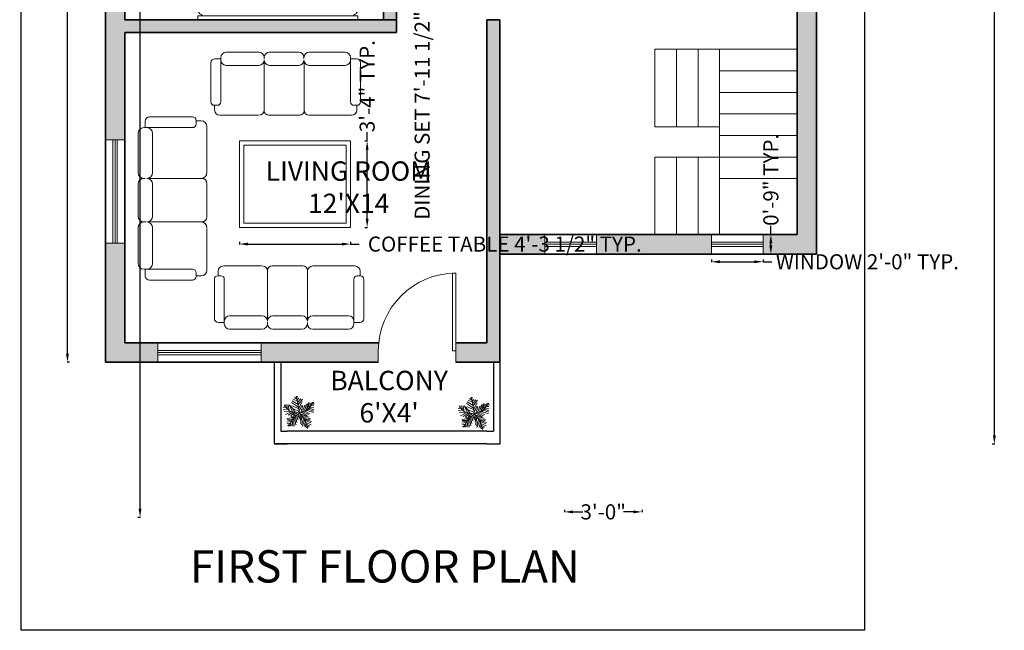
# Model space of a CAD drawing. Units: inches. Extents: x -80 to 1461, y -1239 to 153.
# Tile 4 of 6: x 358 to 815, y -556 to -273. Entities that reach past the tile are written whole.
import ezdxf

# ---------------------------------------------------------------- set-up
doc = ezdxf.new("R2010")
doc.units = ezdxf.units.IN
doc.header["$MEASUREMENT"] = 0
for name, color, linetype, lineweight in [('A-ANNO-DIMS', 2, 'Continuous', 18), ('A-ANNO-TEXT', 7, 'Continuous', 18), ('A-ANNO-TTLB', 7, 'Continuous', 25), ('A-AREA-IDEN', 7, 'Continuous', 18), ('A-FLOR', 7, 'Continuous', 25), ('A-FLOR-STRS', 7, 'Continuous', 20), ('A-FURN', 8, 'Continuous', 18), ('A-GLAZ', 4, 'Continuous', 18), ('A-WALL', 7, 'Continuous', 35), ('A-WALL-PATT', 8, 'Continuous', 13), ('DOOR', 32, 'Continuous', 18), ('TREE', 92, 'Continuous', 13)]:
    doc.layers.add(name, color=color, linetype=linetype, lineweight=lineweight)
doc.styles.get("Standard").update_dxf_attribs({"font": 'arial.ttf'})
doc.dimstyles.get("Standard").update_dxf_attribs({"dimtxt": 7, "dimasz": 4, "dimexe": 0.18, "dimexo": 0.0625, "dimgap": 0.09, "dimtad": 0, "dimdec": 0, "dimzin": 0, "dimdsep": 46, "dimlunit": 3, "dimtxsty": 'Standard', "dimcen": 0.09, "dimadec": 0, "dimazin": 0, "dimtfac": 1, "dimtdec": 0, "dimtofl": 0, "dimtmove": 0, "dimatfit": 3, "dimfxl": 1, "dimfxlon": 1, "dimtolj": 1, "dimtzin": 0, "dimarcsym": 0})

# ---------------------------------------------------------------- blocks, each defined once
blk = doc.blocks.new('*U10')
for p, q in [((-3.665, 19.273), (-27.574, 35.527)), ((-5.114, 28.097), (-24.676, 40.636)), ((-7.288, 39.707), (-21.778, 46.673)), ((-8.737, 47.138), (-17.069, 52.711)), ((-10.186, 53.64), (-13.084, 55.962)), ((0, 0), (-10.5, 57)), ((-9.099, 51.782), (-6.563, 55.962)), ((-7.65, 43.423), (-2.578, 49.46)), ((-5.839, 35.992), (4.667, 48.067)), ((-5.114, 27.632), (10.463, 46.673)), ((-2.941, 16.486), (8.652, 37.85)), ((27, 9), (48, 36)), ((27.127, 9.056), (31.112, 35.992)), ((38.719, 34.134), (41.979, 28.561)), ((44.153, 36.456), (45.239, 32.741)), ((-47.498, 19.737), (-55.83, 18.344)), ((-40.615, 13.7), (-55.105, 10.913)), ((-31.5, 4.5), (-52.5, 25.5)), ((-33.37, 6.269), (-52.207, 5.34)), ((-48.585, 21.131), (-49.309, 29.026)), ((-28.299, 3.483), (-47.86, -5.805)), ((-43.513, 28.561), (-42.427, 15.558)), ((-38.442, 26.239), (-34.819, 7.663)), ((-21.416, 3.018), (-38.079, -8.128)), ((-35.544, 28.097), (-24.314, 3.947)), ((0, 0), (-31.5, 4.5)), ((-14.533, 2.09), (-30.834, 25.31)), ((-15.982, 2.09), (-30.11, -9.521)), ((-24.314, 23.917), (-2.941, 13.7)), ((0, 0), (-22.5, -19.5)), ((-6.563, 1.161), (-21.416, -8.128)), ((-20.691, 13.7), (-1.129, 4.876)), ((-1.129, 6.734), (9.014, 26.704)), ((0, 0), (27, 9)), ((0, 0), (18, -22.5)), ((3.942, 1.625), (11.187, 24.381)), ((6.478, 1.625), (26.04, -8.592)), ((10.101, 3.483), (17.708, 26.239)), ((11.187, 3.483), (30.749, -5.805)), ((16.259, 5.805), (23.142, 31.348)), ((18.07, 5.805), (35.096, -3.483)), ((22.055, 7.198), (27.489, 32.277)), ((24.229, 7.663), (46.688, 1.625)), ((29.662, 12.307), (48.137, 6.269)), ((31.836, 30.883), (32.561, 16.486)), ((33.285, 16.486), (48.862, 10.913)), ((35.096, 32.741), (37.27, 22.524)), ((36.183, 19.737), (48.137, 17.88)), ((40.53, 25.775), (48.862, 24.846)), ((43.791, 29.954), (51.036, 30.883)), ((-17.431, -15.094), (-42.789, -18.809)), ((-28.299, -29.026), (-42.789, -31.348)), ((-24.314, -21.596), (-42.427, -22.06)), ((-26.849, -26.24), (-40.253, -25.775)), ((-22.5, -19.5), (-37.5, -45)), ((-15.257, -12.772), (-30.11, -12.772)), ((-29.023, -30.884), (-27.936, -43.887)), ((-25.038, -23.918), (-22.865, -45.281)), ((-20.691, -18.345), (-17.793, -44.352)), ((-6.563, -5.805), (-19.967, -9.985)), ((-17.069, -15.094), (-12.721, -40.172)), ((-13.446, -11.378), (-8.737, -32.741)), ((-9.461, -8.592), (-6.201, -23.453)), ((-4.752, -3.483), (-3.665, -14.629)), ((2.493, -3.019), (-1.491, -20.202)), ((1.769, -2.555), (24.229, -9.521)), ((5.029, -6.27), (2.131, -25.775)), ((9.014, -11.378), (3.58, -35.992)), ((14.085, -16.951), (6.478, -40.172)), ((7.565, -9.056), (32.198, -14.629)), ((18.07, -22.524), (8.289, -45.745)), ((12.274, -15.094), (36.907, -18.809)), ((20.244, -30.419), (15.897, -44.816)), ((16.259, -19.738), (36.183, -22.989)), ((18, -22.5), (27, -52.5)), ((18.433, -22.524), (40.53, -29.026)), ((19.157, -25.311), (38.719, -33.206)), ((21.331, -32.741), (39.081, -40.636)), ((-30.834, -34.135), (-42.427, -35.528)), ((-34.457, -39.708), (-40.978, -42.494)), ((-32.646, -36.921), (-31.921, -44.352)), ((22.78, -37.85), (19.519, -48.532)), ((22.78, -38.314), (34.372, -44.816)), ((24.591, -45.745), (23.142, -50.854)), ((24.591, -43.423), (30.749, -47.603)), ((26.764, -49.925), (28.213, -50.854))]:
    blk.add_line(p, q)
blk = doc.blocks.new('*U2')
for p, q in [((0, 0), (0, -6)), ((40, 0), (40, -6))]:
    blk.add_line(p, q)
blk.add_lwpolyline([(0, 0), (0, 40), (1.75, 40), (1.75, 0)], close=True)
blk.add_arc((0, 0), 40, 0, 90)
blk = doc.blocks.new('A$C164346CA')
for p, q in [((0, 2.035), (0, 2)), ((1.5, 2.035), (0, 2.035)), ((1.5, 2), (1.5, 2.035)), ((1.5, 2), (0, 2)), ((0, 1.93), (0, 0.07)), ((0.0919, 1.8624), (0.0919, 1.6069)), ((0.6731, 1.9024), (0.1319, 1.9024)), ((0.7131, 1.6069), (0.7131, 1.8624)), ((0.7828, 1.8624), (0.7828, 1.6069)), ((1.364, 1.9024), (0.8228, 1.9024)), ((1.404, 1.6069), (1.404, 1.8624)), ((1.5, 0.07), (1.5, 1.93)), ((0.1319, 1.5669), (0.6731, 1.5669)), ((0.8228, 1.5669), (1.364, 1.5669)), ((0.8395, 1.4761), (0, 1.4761)), ((0.8395, 1.4761), (1.2448, 1.12)), ((1.5, 1.2611), (0.8395, 1.4761)), ((1.3077, 1.1175), (1.5, 1.2611)), ((0.07, 0), (1.43, 0))]:
    blk.add_line(p, q)
for centre, radius, start, end in [((0.07, 1.93), 0.07, 90, 180), ((1.43, 1.93), 0.07, 0, 90), ((0.1319, 1.8624), 0.04, 90, 180), ((0.6731, 1.8624), 0.04, 0, 90), ((0.8228, 1.8624), 0.04, 90, 180), ((1.364, 1.8624), 0.04, 0, 90), ((0.1319, 1.6069), 0.04, 180, 270), ((0.6731, 1.6069), 0.04, 270, 0), ((0.8228, 1.6069), 0.04, 180, 270), ((1.364, 1.6069), 0.04, 270, 0), ((1.2778, 1.1575), 0.05, 228.69584, 306.75789), ((0.07, 0.07), 0.07, 180, 270), ((1.43, 0.07), 0.07, 270, 0)]:
    blk.add_arc(centre, radius, start, end)
blk = doc.blocks.new('A$C0876780F')
for p, q in [((0.72, 0.95), (0.23, 0.95)), ((1.32, 0.95), (0.88, 0.95)), ((1.48, 0.95), (2.02, 0.95)), ((0.15, 0.85), (0.06, 0.85)), ((0.15, 0.87), (0.15, 0.844)), ((0.15, 0.87), (0.15, 0.85)), ((0.15, 0.21), (0.15, 0.85)), ((0.8, 0.85), (0.8, 0.87)), ((0.8, 0.87), (0.8, 0.85)), ((0.8, 0.87), (0.8, 0.844)), ((0.801, 0.82), (0.801, 0.08)), ((1.4, 0.85), (1.4, 0.87)), ((1.4, 0.85), (1.4, 0.87)), ((2.1, 0.87), (2.1, 0.85)), ((2.1, 0.87), (2.1, 0.844)), ((2.1, 0.21), (2.1, 0.85)), ((2.1, 0.85), (2.19, 0.85)), ((0, 0.79), (0, 0.21)), ((0.72, 0.75), (0.23, 0.75)), ((1.32, 0.75), (0.88, 0.75)), ((1.401, 0.08), (1.401, 0.803)), ((1.48, 0.75), (2.02, 0.75)), ((2.25, 0.79), (2.25, 0.21)), ((0, 0.21), (0, 0.2)), ((0.05, 0.15), (0.1, 0.15)), ((0.056, 0.15), (0.056, 0.08)), ((0.15, 0.2), (0.15, 0.25)), ((2.1, 0.2), (2.1, 0.25)), ((2.2, 0.15), (2.15, 0.15)), ((2.194, 0.15), (2.194, 0.08)), ((2.25, 0.21), (2.25, 0.2)), ((0.136, 0), (0.709, 0)), ((0.801, 0.07), (0.801, 0.08)), ((0.871, 0), (1.331, 0)), ((1.401, 0.07), (1.401, 0.08)), ((2.114, 0), (1.48, 0))]:
    blk.add_line(p, q)
for centre, radius, start, end in [((0.23, 0.87), 0.08, 90, 180), ((0.72, 0.87), 0.08, 0, 90), ((0.88, 0.87), 0.08, 90, 180), ((1.32, 0.87), 0.08, 0, 90), ((1.48, 0.87), 0.08, 90, 180), ((2.02, 0.87), 0.08, 0, 90), ((0.06, 0.79), 0.06, 90, 180), ((0.23, 0.83), 0.08, 180, 270), ((0.23, 0.83), 0.08, 180, 270), ((0.72, 0.83), 0.08, 270, 0), ((0.88, 0.83), 0.08, 180, 270), ((0.88, 0.83), 0.08, 180, 270), ((1.32, 0.83), 0.08, 270, 0), ((1.48, 0.83), 0.08, 180, 270), ((2.02, 0.83), 0.08, 270, 0), ((2.02, 0.83), 0.08, 270, 0), ((2.19, 0.79), 0.06, 0, 90), ((0.05, 0.2), 0.05, 180, 270), ((0.1, 0.2), 0.05, 270, 0), ((0.09, 0.21), 0.06, 350.5377, 0), ((2.16, 0.21), 0.06, 180, 189.4623), ((2.15, 0.2), 0.05, 180, 270), ((2.2, 0.2), 0.05, 270, 0), ((0.136, 0.08), 0.08, 180, 270), ((0.721, 0.08), 0.08, 270, 0), ((0.871, 0.07), 0.07, 180, 270), ((1.331, 0.07), 0.07, 270, 0), ((1.481, 0.08), 0.08, 180, 270), ((2.114, 0.08), 0.08, 270, 0)]:
    blk.add_arc(centre, radius, start, end)
blk = doc.blocks.new('*D14')
at = {"layer": 'A-ANNO-DIMS', "color": 0, "lineweight": -2, "transparency": 16777216}
for p, q in [((380.82, 30.32), (379.64, 30.32)), ((379.82, 26.32), (379.82, -188.57)), ((379.82, -427.68), (379.82, -212.8)), ((380.82, -431.68), (379.64, -431.68))]:
    blk.add_line(p, q, dxfattribs=at)
at = {"layer": 'A-ANNO-DIMS', "color": 0, "transparency": 16777216}
for points in [[(379.15, 26.32), (380.48, 26.32), (379.82, 30.32)], [(379.15, -427.68), (380.48, -427.68), (379.82, -431.68)]]:
    blk.add_solid(points, dxfattribs=at)
at = {"layer": 'Defpoints', "color": 0, "transparency": 16777216}
for p in [(397.42, 30.32), (379.82, -431.68), (397.42, -431.68)]:
    blk.add_point(p, dxfattribs=at)
at = {"layer": 'A-ANNO-DIMS', "color": 0, "transparency": 16777216, "insert": (379.82, -200.68), "char_height": 7, "attachment_point": 5, "rotation": 90}
blk.add_mtext('\\A1;38\'-6"', dxfattribs=at)
blk = doc.blocks.new('WIN-48IN')
for p, q in [((0, 9), (0, 0)), ((48, 9), (0, 9)), ((0, 5.5), (48, 5.5)), ((48, 0), (48, 9)), ((0, 4.5), (48, 4.5)), ((0, 3.5), (48, 3.5)), ((0, 0), (36, 0)), ((36, 0), (48, 0))]:
    blk.add_line(p, q)
blk = doc.blocks.new('WIN-24IN')
for p, q in [((0, 9), (0, 0)), ((0, 9), (24, 9)), ((0, 5.5), (24, 5.5)), ((24, 9), (24, 0)), ((0, 4.5), (24, 4.5)), ((0, 3.5), (24, 3.5)), ((0, 0), (24, 0))]:
    blk.add_line(p, q)
blk = doc.blocks.new('COFFEE-TABLE')
for points in [[(0, 40.15), (51.49, 40.15), (51.49, 0), (0, 0)], [(2, 38.15), (49.49, 38.15), (49.49, 2), (2, 2)]]:
    blk.add_lwpolyline(points, close=True)
blk = doc.blocks.new('STAIR-RETURN-PLAN')
for p, q in [((0, 86), (0, 50)), ((0, 86), (30, 86)), ((10, 86), (10, 50)), ((20, 86), (20, 50)), ((66, 86), (30, 86)), ((30, 86), (30, 50)), ((66, 76), (30, 76)), ((66, 66), (30, 66)), ((66, 56), (30, 56)), ((0, 50), (30, 50)), ((30, 50), (30, 36)), ((66, 46), (30, 46)), ((0, 36), (0, 0)), ((0, 36), (30, 36)), ((10, 36), (10, 0)), ((20, 36), (20, 0)), ((66, 36), (30, 36)), ((30, 36), (30, 0)), ((66, 26), (30, 26))]:
    blk.add_line(p, q)
blk = doc.blocks.new('*D38')
at = {"layer": 'A-ANNO-DIMS', "color": 0, "lineweight": -2, "transparency": 16777216}
for p, q in [((678.59, -384.02), (678.59, -385.2)), ((682.59, -385.02), (698.59, -385.02)), ((702.59, -384.02), (702.59, -385.2)), ((702.59, -385.02), (706.59, -385.02))]:
    blk.add_line(p, q, dxfattribs=at)
at = {"layer": 'A-ANNO-DIMS', "color": 0, "transparency": 16777216}
for points in [[(682.59, -384.36), (682.59, -385.69), (678.59, -385.02)], [(698.59, -384.36), (698.59, -385.69), (702.59, -385.02)]]:
    blk.add_solid(points, dxfattribs=at)
at = {"layer": 'Defpoints', "color": 0, "transparency": 16777216}
for p in [(678.59, -381.42), (702.59, -381.42), (702.59, -385.02)]:
    blk.add_point(p, dxfattribs=at)
at = {"layer": 'A-ANNO-DIMS', "color": 0, "transparency": 16777216, "insert": (750.97, -385.02), "char_height": 7, "attachment_point": 5}
blk.add_mtext('\\A1;WINDOW 2\'-0" TYP.', dxfattribs=at)
blk = doc.blocks.new('*D39')
at = {"layer": 'A-ANNO-DIMS', "color": 0, "lineweight": -2, "transparency": 16777216}
for p, q in [((706.19, -372.42), (706.19, -368.42)), ((705.19, -372.42), (706.37, -372.42)), ((706.19, -377.42), (706.19, -376.42)), ((705.19, -381.42), (706.37, -381.42))]:
    blk.add_line(p, q, dxfattribs=at)
at = {"layer": 'A-ANNO-DIMS', "color": 0, "transparency": 16777216}
for points in [[(705.52, -376.42), (706.86, -376.42), (706.19, -372.42)], [(705.52, -377.42), (706.86, -377.42), (706.19, -381.42)]]:
    blk.add_solid(points, dxfattribs=at)
at = {"layer": 'Defpoints', "color": 0, "transparency": 16777216}
for p in [(702.59, -372.42), (706.19, -372.42), (702.59, -381.42)]:
    blk.add_point(p, dxfattribs=at)
at = {"layer": 'A-ANNO-DIMS', "color": 0, "transparency": 16777216, "insert": (706.19, -347), "char_height": 7, "attachment_point": 5, "rotation": 90}
blk.add_mtext('\\A1;0\'-9" TYP.', dxfattribs=at)
blk = doc.blocks.new('*D52')
at = {"layer": 'A-ANNO-DIMS', "color": 0, "lineweight": -2, "transparency": 16777216}
for p, q in [((545.39, -145.12), (544.21, -145.12)), ((544.39, -149.12), (544.39, -236.86)), ((545.39, -240.86), (544.21, -240.86)), ((544.39, -240.86), (544.39, -244.86))]:
    blk.add_line(p, q, dxfattribs=at)
at = {"layer": 'A-ANNO-DIMS', "color": 0, "transparency": 16777216}
for points in [[(543.72, -149.12), (545.06, -149.12), (544.39, -145.12)], [(543.72, -236.86), (545.06, -236.86), (544.39, -240.86)]]:
    blk.add_solid(points, dxfattribs=at)
at = {"layer": 'Defpoints', "color": 0, "transparency": 16777216}
for p in [(558.75, -145.12), (544.39, -240.86), (558.75, -240.86)]:
    blk.add_point(p, dxfattribs=at)
at = {"layer": 'A-ANNO-DIMS', "color": 0, "transparency": 16777216, "insert": (544.39, -306.33), "char_height": 7, "attachment_point": 5, "rotation": 90}
blk.add_mtext('\\A1;DINING SET 7\'-11 1/2" TYP.', dxfattribs=at)
blk = doc.blocks.new('*D54')
at = {"layer": 'A-ANNO-DIMS', "color": 0, "lineweight": -2, "transparency": 16777216}
for p, q in [((459.66, -375.81), (459.66, -376.99)), ((463.66, -376.81), (507.15, -376.81)), ((511.15, -375.81), (511.15, -376.99)), ((511.15, -376.81), (515.15, -376.81))]:
    blk.add_line(p, q, dxfattribs=at)
at = {"layer": 'A-ANNO-DIMS', "color": 0, "transparency": 16777216}
for points in [[(463.66, -376.15), (463.66, -377.48), (459.66, -376.81)], [(507.15, -376.15), (507.15, -377.48), (511.15, -376.81)]]:
    blk.add_solid(points, dxfattribs=at)
at = {"layer": 'Defpoints', "color": 0, "transparency": 16777216}
for p in [(459.66, -369.09), (511.15, -369.09), (511.15, -376.81)]:
    blk.add_point(p, dxfattribs=at)
at = {"layer": 'A-ANNO-DIMS', "color": 0, "transparency": 16777216, "insert": (582.73, -376.81), "char_height": 7, "attachment_point": 5}
blk.add_mtext('\\A1;COFFEE TABLE 4\'-3 1/2" TYP.', dxfattribs=at)
blk = doc.blocks.new('*D55')
at = {"layer": 'A-ANNO-DIMS', "color": 0, "lineweight": -2, "transparency": 16777216}
for p, q in [((517.87, -328.94), (519.05, -328.94)), ((518.87, -328.94), (518.87, -324.94)), ((518.87, -365.09), (518.87, -332.94)), ((517.87, -369.09), (519.05, -369.09))]:
    blk.add_line(p, q, dxfattribs=at)
at = {"layer": 'A-ANNO-DIMS', "color": 0, "transparency": 16777216}
for points in [[(518.21, -332.94), (519.54, -332.94), (518.87, -328.94)], [(518.21, -365.09), (519.54, -365.09), (518.87, -369.09)]]:
    blk.add_solid(points, dxfattribs=at)
at = {"layer": 'Defpoints', "color": 0, "transparency": 16777216}
for p in [(511.15, -328.94), (518.87, -328.94), (511.15, -369.09)]:
    blk.add_point(p, dxfattribs=at)
at = {"layer": 'A-ANNO-DIMS', "color": 0, "transparency": 16777216, "insert": (518.87, -303.51), "char_height": 7, "attachment_point": 5, "rotation": 90}
blk.add_mtext('\\A1;3\'-4" TYP.', dxfattribs=at)
blk = doc.blocks.new('*D72')
at = {"layer": 'A-ANNO-DIMS', "color": 0, "lineweight": -2, "transparency": 16777216}
for p, q in [((412.49, 30.32), (413.67, 30.32)), ((413.49, 26.32), (413.49, -224.38)), ((413.49, -499.58), (413.49, -248.89)), ((412.49, -503.58), (413.67, -503.58))]:
    blk.add_line(p, q, dxfattribs=at)
at = {"layer": 'A-ANNO-DIMS', "color": 0, "transparency": 16777216}
for points in [[(412.82, 26.32), (414.16, 26.32), (413.49, 30.32)], [(412.82, -499.58), (414.16, -499.58), (413.49, -503.58)]]:
    blk.add_solid(points, dxfattribs=at)
at = {"layer": 'Defpoints', "color": 0, "transparency": 16777216}
for p in [(330.99, 30.32), (183.99, -503.58), (413.49, -503.58)]:
    blk.add_point(p, dxfattribs=at)
at = {"layer": 'A-ANNO-DIMS', "color": 0, "transparency": 16777216, "insert": (413.49, -236.63), "char_height": 7, "attachment_point": 5, "rotation": 90}
blk.add_mtext('\\A1;44\'-6"', dxfattribs=at)
blk = doc.blocks.new('*D73')
at = {"layer": 'A-ANNO-DIMS', "color": 0, "lineweight": -2, "transparency": 16777216}
for p, q in [((808.92, 30.32), (810.1, 30.32)), ((809.92, 26.32), (809.92, -207.38)), ((809.92, -465.58), (809.92, -231.89)), ((808.92, -469.58), (810.1, -469.58))]:
    blk.add_line(p, q, dxfattribs=at)
at = {"layer": 'A-ANNO-DIMS', "color": 0, "transparency": 16777216}
for points in [[(809.25, 26.32), (810.58, 26.32), (809.92, 30.32)], [(809.25, -465.58), (810.58, -465.58), (809.92, -469.58)]]:
    blk.add_solid(points, dxfattribs=at)
at = {"layer": 'Defpoints', "color": 0, "transparency": 16777216}
for p in [(727.42, 30.32), (809.92, 30.32), (580.42, -469.58)]:
    blk.add_point(p, dxfattribs=at)
at = {"layer": 'A-ANNO-DIMS', "color": 0, "transparency": 16777216, "insert": (809.92, -219.63), "char_height": 7, "attachment_point": 5, "rotation": 90}
blk.add_mtext('\\A1;41\'-8"', dxfattribs=at)
blk = doc.blocks.new('*D77')
at = {"layer": 'A-ANNO-DIMS', "color": 0, "lineweight": -2, "transparency": 16777216}
for p, q in [((610.42, -500.08), (610.42, -501.26)), ((614.42, -501.08), (619.02, -501.08)), ((642.42, -501.08), (637.81, -501.08)), ((646.42, -500.08), (646.42, -501.26))]:
    blk.add_line(p, q, dxfattribs=at)
at = {"layer": 'A-ANNO-DIMS', "color": 0, "transparency": 16777216}
for points in [[(614.42, -500.42), (614.42, -501.75), (610.42, -501.08)], [(642.42, -500.42), (642.42, -501.75), (646.42, -501.08)]]:
    blk.add_solid(points, dxfattribs=at)
at = {"layer": 'Defpoints', "color": 0, "transparency": 16777216}
for p in [(610.42, -104.68), (646.42, -104.68), (646.42, -501.08)]:
    blk.add_point(p, dxfattribs=at)
at = {"layer": 'A-ANNO-DIMS', "color": 0, "transparency": 16777216, "insert": (628.42, -501.08), "char_height": 7, "attachment_point": 5}
blk.add_mtext('\\A1;3\'-0"', dxfattribs=at)

msp = doc.modelspace()

# ---------------------------------------------------------------- hatches: boundary and pattern name
at = {"layer": 'A-WALL-PATT'}
h = msp.add_hatch(color=256, dxfattribs=at)
h.dxf.hatch_style = 1
h.paths.add_polyline_path([(558.8, 30.32), (495.28, 30.32), (495.28, 21.32), (538.42, 21.32), (538.42, -81.2, -0.004167), (539.02, -81.2), (544.42, -81.2), (544.42, 21.32), (558.8, 21.32)])
h.paths.add_polyline_path([(727.42, 30.32), (693.99, 30.32), (693.99, 21.32), (718.42, 21.32), (718.42, -3.69), (727.42, -3.69)])
h.paths.add_polyline_path([(645.99, 30.32), (582.8, 30.32), (582.8, 21.32), (588.82, 21.32), (604.42, 21.32), (604.42, -104.68), (610.42, -104.68), (610.42, -99.28), (610.42, -63.28), (610.42, 21.32), (645.99, 21.32)])
h.paths.add_polyline_path([(727.42, -39.69), (718.42, -39.69), (718.42, -98.68), (646.41, -98.68, -0.004167), (646.42, -99.28), (646.42, -104.68), (718.42, -104.68), (718.42, -132.06), (727.42, -132.06)])
h.paths.add_polyline_path([(727.42, -156.06), (718.42, -156.06), (718.42, -166.56), (718.42, -188.68), (658.42, -188.68), (658.42, -133.64, -0.014233), (656.77, -133.68), (652.42, -133.68), (652.42, -194.68), (718.42, -194.68), (718.42, -372.42), (702.59, -372.42), (702.59, -381.42), (727.42, -381.42)])
h = msp.add_hatch(color=256, dxfattribs=at)
h.dxf.hatch_style = 1
h.paths.add_polyline_path([(580.42, -272.68), (574.42, -272.68), (574.42, -422.68), (560.05, -422.68), (560.05, -426.28), (560.05, -431.68), (580.42, -431.68)])
h.paths.add_polyline_path([(406.42, -220.33), (397.42, -220.33), (397.42, -328.45), (406.42, -328.45), (406.42, -278.68), (532.42, -278.68), (532.42, -272.68), (406.42, -272.68)])
h.paths.add_polyline_path([(532.42, -164.68), (527.02, -164.68, -0.004167), (526.42, -164.68), (526.42, -272.68), (532.42, -272.68)])
h.paths.add_polyline_path([(524.05, -426.28, -0.025047), (524.23, -422.68), (469.7, -422.68), (469.7, -431.68), (524.05, -431.68)])
h.paths.add_polyline_path([(421.7, -422.68), (406.42, -422.68), (406.42, -376.45), (397.42, -376.45), (397.42, -431.68), (421.7, -431.68)])
h = msp.add_hatch(color=256, dxfattribs=at)
h.dxf.hatch_style = 1
h.paths.add_polyline_path([(678.59, -372.42), (625.36, -372.42), (625.36, -381.42), (678.59, -381.42)])
h.paths.add_polyline_path([(601.36, -372.42), (580.42, -372.42), (580.42, -381.42), (601.36, -381.42)])

# ---------------------------------------------------------------- linework, layer by layer
at = {"layer": 'A-ANNO-TTLB'}
msp.add_lwpolyline([(358.28, 71.88), (749.61, 71.88), (749.61, -556.04), (358.28, -556.04)], close=True, dxfattribs=at)
at = {"layer": 'A-FLOR'}
for p, q in [((475.79, -431.68), (475.79, -469.58)), ((478.79, -431.68), (478.79, -463.58)), ((577.42, -431.68), (577.42, -463.58)), ((580.42, -431.68), (580.42, -469.58)), ((478.79, -463.58), (481.79, -463.58)), ((574.42, -463.58), (481.79, -463.58)), ((574.42, -463.58), (577.42, -463.58)), ((574.42, -469.58), (475.79, -469.58)), ((475.79, -469.58), (481.79, -469.58)), ((574.42, -469.58), (580.42, -469.58))]:
    msp.add_line(p, q, dxfattribs=at)
at = {"layer": 'A-WALL'}
for p, q in [((397.42, 30.32), (397.42, -431.68)), ((727.42, 30.32), (727.42, -381.42)), ((406.42, -128.68), (406.42, -272.68)), ((526.42, -164.68), (526.42, -272.68)), ((532.42, -164.68), (532.42, -278.68)), ((718.42, -194.68), (718.42, -372.42)), ((406.42, -272.68), (532.42, -272.68)), ((574.42, -272.68), (580.42, -272.68)), ((574.42, -272.68), (574.42, -422.68)), ((580.42, -272.68), (580.42, -431.68)), ((406.42, -278.68), (532.42, -278.68)), ((406.42, -278.68), (406.42, -422.68)), ((580.42, -372.42), (718.42, -372.42)), ((580.42, -381.42), (727.42, -381.42)), ((406.42, -422.68), (524.23, -422.68)), ((560.05, -422.68), (574.42, -422.68)), ((397.42, -431.68), (524.05, -431.68)), ((560.05, -431.68), (580.42, -431.68))]:
    msp.add_line(p, q, dxfattribs=at)

# ---------------------------------------------------------------- block references
at = {"layer": 'A-FLOR-STRS'}
msp.add_blockref('STAIR-RETURN-PLAN', (652.42, -372.42), dxfattribs=at)
at = {"layer": 'A-FURN'}
for name, p, xscale, yscale, zscale, rotation in [('A$C164346CA', (514.6, -171.81), 49.56739756478314, 49.56739756478314, 49.56739756478314, 180), ('A$C0876780F', (444.56, -393.5), 33.67837588954761, 33.67837588954761, 33.67837588954761, 90), ('A$C0876780F', (447.97, -386.96), -30.83775321962601, 30.83775321962601, 30.83775321962601, 180)]:
    msp.add_blockref(name, p, dxfattribs=dict(at, xscale=xscale, yscale=yscale, zscale=zscale, rotation=rotation))
at = {"layer": 'A-FURN', "xscale": 30.83775321962601, "yscale": 30.83775321962601, "zscale": 30.83775321962601}
msp.add_blockref('A$C0876780F', (446.39, -317.03), dxfattribs=at)
at = {"layer": 'A-FURN'}
msp.add_blockref('COFFEE-TABLE', (459.66, -369.09), dxfattribs=at)
at = {"layer": 'A-GLAZ', "rotation": 90.00000000000011}
msp.add_blockref('WIN-48IN', (406.42, -376.45), dxfattribs=at)
at = {"layer": 'A-GLAZ'}
for name, p in [('WIN-24IN', (601.36, -381.42)), ('WIN-24IN', (678.59, -381.42)), ('WIN-48IN', (421.7, -431.68))]:
    msp.add_blockref(name, p, dxfattribs=at)
at = {"layer": 'DOOR', "xscale": -0.9, "yscale": 0.9, "zscale": 0.9}
msp.add_blockref('*U2', (560.05, -426.28), dxfattribs=at)
at = {"layer": 'TREE', "xscale": 0.1370045651508197, "yscale": 0.1370045651508197, "zscale": 0.1370045651508197}
for p in [(487.51, -455.16), (568.7, -455.64)]:
    msp.add_blockref('*U10', p, dxfattribs=at)

# ---------------------------------------------------------------- texts
at = {"layer": 'A-ANNO-TEXT', "insert": (404.58, -518.87), "char_height": 15, "attachment_point": 1}
msp.add_mtext_dynamic_manual_height_columns('\\pxqc;FIRST FLOOR PLAN', width=245.0183, gutter_width=1, heights=[0], dxfattribs=at)
at = {"layer": 'A-AREA-IDEN', "char_height": 9, "attachment_point": 1}
for s, insert in [("\\pxqc;LIVING ROOM\\P12'X14", (461.94, -338.43)), ("\\pxqc;BALCONY\\P6'X4'", (480.69, -435.6))]:
    msp.add_mtext_dynamic_manual_height_columns(s, width=96.7224, gutter_width=1, heights=[0], dxfattribs=dict(at, insert=insert))

# ---------------------------------------------------------------- dimensions: what is measured, and where the dimension line sits
at = {"layer": 'A-ANNO-DIMS'}
for base, p1, p2, override, picture, middle in [((413.49, -503.58), (330.99, 30.32), (183.99, -503.58), {"dimdec": 1, "dimlfac": 1, "dimrnd": 0, "dimzin": 1, "dimdsep": 46, "dimlunit": 4, "dimfrac": 2}, '*D72', (413.49, -236.63)), ((379.82, -431.68), (397.42, 30.32), (397.42, -431.68), {"dimclrd": 0, "dimclre": 0, "dimclrt": 0}, '*D14', (379.82, -200.68)), ((809.92, 30.32), (580.42, -469.58), (727.42, 30.32), {"dimdec": 1, "dimlfac": 1, "dimrnd": 0, "dimzin": 1, "dimdsep": 46, "dimlunit": 4, "dimfrac": 2}, '*D73', (809.92, -219.63))]:
    dim = msp.add_linear_dim(base=base, p1=p1, p2=p2, angle=90, dimstyle='Standard', override=override, dxfattribs=at)
    dim.commit()
    dim.dimension.update_dxf_attribs({"geometry": picture, "text_midpoint": middle})
dim = msp.add_linear_dim(base=(646.42, -501.08), p1=(610.42, -104.68), p2=(646.42, -104.68), dimstyle='Standard', override={"dimdec": 1, "dimlfac": 1, "dimrnd": 0, "dimzin": 1, "dimdsep": 46, "dimlunit": 4, "dimfrac": 2}, dxfattribs=at)
dim.commit()
dim.dimension.update_dxf_attribs({"geometry": '*D77', "text_midpoint": (628.42, -501.08)})
for base, p1, p2, angle, text, picture, middle in [((544.39, -240.86), (558.75, -145.12), (558.75, -240.86), 270, 'DINING SET <> TYP.', '*D52', (544.39, -306.33)), ((518.8745, -328.9363), (511.1515, -369.0888), (511.1515, -328.9363), 90, '<> TYP.', '*D55', (518.8745, -303.5144)), ((706.19, -372.42), (702.59, -381.42), (702.59, -372.42), 90, '<> TYP.', '*D39', (706.19, -347))]:
    dim = msp.add_linear_dim(base=base, p1=p1, p2=p2, angle=angle, text=text, dimstyle='Standard', override={"dimdec": 1, "dimlfac": 1, "dimrnd": 0, "dimzin": 1, "dimdsep": 46, "dimlunit": 4, "dimfrac": 2}, dxfattribs=at)
    dim.commit()
    dim.dimension.update_dxf_attribs({"geometry": picture, "text_midpoint": middle})
for base, p1, p2, text, picture, middle in [((511.15, -376.81), (459.66, -369.09), (511.15, -369.09), 'COFFEE TABLE <> TYP.', '*D54', (582.73, -376.81)), ((702.59, -385.02), (678.59, -381.42), (702.59, -381.42), 'WINDOW <> TYP.', '*D38', (750.97, -385.02))]:
    dim = msp.add_linear_dim(base=base, p1=p1, p2=p2, text=text, dimstyle='Standard', override={"dimdec": 1, "dimlfac": 1, "dimrnd": 0, "dimzin": 1, "dimdsep": 46, "dimlunit": 4, "dimfrac": 2}, dxfattribs=at)
    dim.commit()
    dim.dimension.update_dxf_attribs({"geometry": picture, "text_midpoint": middle})

doc.saveas('drawing.dxf')
